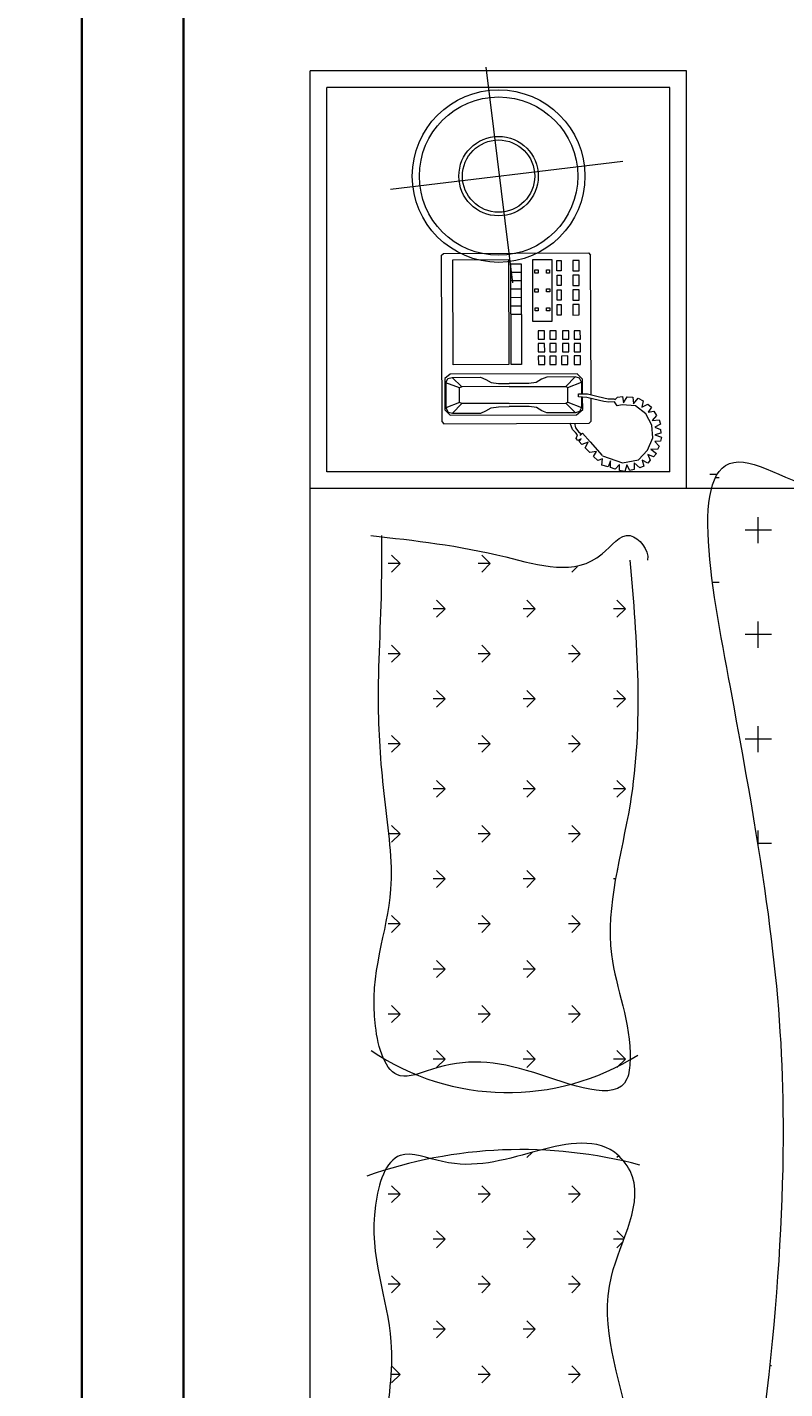
# Model space of a CAD drawing. Units: inches. Extents: x 3731 to 4318, y 1310 to 2388.
# Tile 36 of 57: x 3833 to 3870, y 2243 to 2310. Entities that reach past the tile are written whole.
import ezdxf

# ---------------------------------------------------------------- set-up
doc = ezdxf.new("R2010")
doc.units = ezdxf.units.IN
for name, color, linetype, lineweight in [('A-ANNO-DIMS', 2, 'Continuous', 18), ('A-FURN', 8, 'Continuous', 13), ('A-WALL', 7, 'Continuous', 35)]:
    doc.layers.add(name, color=color, linetype=linetype, lineweight=lineweight)
doc.styles.get("Standard").update_dxf_attribs({"font": 'arial.ttf'})
doc.dimstyles.get("Standard").update_dxf_attribs({"dimtxt": 0.18, "dimasz": 0.18, "dimexe": 0.18, "dimexo": 0.0625, "dimgap": 0.09, "dimtad": 0, "dimtih": 1, "dimtoh": 1, "dimdec": 4, "dimzin": 0, "dimdsep": 46, "dimtxsty": 'Standard', "dimcen": 0.09, "dimadec": 0, "dimazin": 0, "dimtfac": 1, "dimtdec": 4, "dimtofl": 0, "dimtmove": 0, "dimatfit": 3, "dimfxl": 1, "dimtolj": 1, "dimtzin": 0, "dimarcsym": 0})

# ---------------------------------------------------------------- blocks, each defined once
blk = doc.blocks.new('A$C200C7901')
for p, q in [((0.5, 2.3334), (2, 2.3334)), ((2, 2.3334), (2.5, 2.3334)), ((2, 1.6055), (2, 2.3334)), ((2.5, 1.8834), (2.5, 2.3334)), ((0.9943, 2.1721), (0.9842, 2.1822)), ((0.9943, 2.1721), (0.9842, 2.1822)), ((1.3176, 2.1721), (1.3075, 2.1822)), ((1.3176, 2.1721), (1.3075, 2.1822)), ((0.9943, 2.0643), (0.9842, 2.0744)), ((0.9943, 2.0643), (0.9842, 2.0744)), ((1.206, 2.0681), (1.1997, 2.0744)), ((1.206, 2.0681), (1.1997, 2.0744)), ((1.2019, 1.9645), (1.1997, 1.9666)), ((1.2019, 1.9645), (1.1997, 1.9666)), ((2, 1.8834), (2.5, 1.8834)), ((2.0129, 1.8445), (2.0129, 1.849)), ((2.0129, 1.8445), (2.0129, 1.849)), ((2.0171, 1.8467), (2.0171, 1.8556)), ((2.0171, 1.8467), (2.0171, 1.8556))]:
    blk.add_line(p, q)
at = {"linetype": 'ByBlock'}
for p, q in [((2.02, 2.3134), (2.48, 2.3134)), ((2.02, 1.9034), (2.02, 2.3134)), ((2.48, 1.9034), (2.48, 2.3134)), ((0.9404, 2.2259), (0.9303, 2.236)), ((0.9404, 2.2259), (0.9303, 2.236)), ((0.9404, 2.2259), (0.9404, 2.2369)), ((0.9404, 2.2259), (0.9404, 2.2369)), ((0.9404, 2.2259), (0.9505, 2.236)), ((0.9404, 2.2259), (0.9505, 2.236)), ((1.0482, 2.2259), (1.0381, 2.236)), ((1.0482, 2.2259), (1.0381, 2.236)), ((1.0482, 2.2259), (1.0482, 2.2402)), ((1.0482, 2.2259), (1.0482, 2.2402)), ((1.0482, 2.2259), (1.0583, 2.236)), ((1.0482, 2.2259), (1.0583, 2.236)), ((1.1559, 2.2259), (1.1458, 2.236)), ((1.1559, 2.2259), (1.1458, 2.236)), ((1.1559, 2.2259), (1.1559, 2.2402)), ((1.1559, 2.2259), (1.1559, 2.2402)), ((1.1559, 2.2259), (1.166, 2.236)), ((1.1559, 2.2259), (1.166, 2.236)), ((1.3714, 2.2259), (1.3613, 2.236)), ((1.3714, 2.2259), (1.3613, 2.236)), ((1.3714, 2.2259), (1.3714, 2.2402)), ((1.3714, 2.2259), (1.3714, 2.2402)), ((1.3714, 2.2259), (1.3815, 2.236)), ((1.3714, 2.2259), (1.3815, 2.236)), ((1.4792, 2.2259), (1.4691, 2.236)), ((1.4792, 2.2259), (1.4691, 2.236)), ((1.4792, 2.2259), (1.4792, 2.2402)), ((1.4792, 2.2259), (1.4792, 2.2402)), ((1.4792, 2.2259), (1.4893, 2.236)), ((1.4792, 2.2259), (1.4893, 2.236)), ((1.587, 2.2259), (1.5769, 2.236)), ((1.587, 2.2259), (1.5769, 2.236)), ((1.587, 2.2259), (1.587, 2.2393)), ((1.587, 2.2259), (1.587, 2.2393)), ((1.587, 2.2259), (1.5971, 2.236)), ((1.587, 2.2259), (1.5971, 2.236)), ((1.6947, 2.2259), (1.6846, 2.236)), ((1.6947, 2.2259), (1.6846, 2.236)), ((1.6947, 2.2259), (1.6947, 2.2402)), ((1.6947, 2.2259), (1.6947, 2.2402)), ((1.6947, 2.2259), (1.7048, 2.236)), ((1.6947, 2.2259), (1.7048, 2.236)), ((1.8025, 2.2259), (1.7924, 2.236)), ((1.8025, 2.2259), (1.7924, 2.236)), ((1.8025, 2.2259), (1.8025, 2.2402)), ((1.8025, 2.2259), (1.8025, 2.2402)), ((1.8025, 2.2259), (1.8126, 2.236)), ((1.8025, 2.2259), (1.8126, 2.236)), ((1.9103, 2.2259), (1.9002, 2.236)), ((1.9103, 2.2259), (1.9002, 2.236)), ((1.9103, 2.2259), (1.9103, 2.2402)), ((1.9103, 2.2259), (1.9103, 2.2402)), ((1.9103, 2.2259), (1.9204, 2.236)), ((1.9103, 2.2259), (1.9204, 2.236)), ((2.3581, 2.2373), (2.3919, 1.9595)), ((0.9943, 2.172), (0.9943, 2.1863)), ((0.9943, 2.172), (0.9943, 2.1863)), ((1.102, 2.172), (1.102, 2.1863)), ((1.102, 2.172), (1.102, 2.1863)), ((1.3176, 2.172), (1.3176, 2.1863)), ((1.3176, 2.172), (1.3176, 2.1863)), ((1.4253, 2.172), (1.4253, 2.1863)), ((1.4253, 2.172), (1.4253, 2.1863)), ((1.5331, 2.172), (1.5331, 2.1863)), ((1.5331, 2.172), (1.5331, 2.1863)), ((1.6408, 2.172), (1.6408, 2.1863)), ((1.6408, 2.172), (1.6408, 2.1863)), ((1.7486, 2.172), (1.7486, 2.1863)), ((1.7486, 2.172), (1.7486, 2.1863)), ((1.8564, 2.172), (1.8564, 2.1863)), ((1.8564, 2.172), (1.8564, 2.1863)), ((0.9943, 2.1721), (1.0044, 2.1822)), ((0.9943, 2.1721), (1.0044, 2.1822)), ((1.102, 2.1721), (1.0919, 2.1822)), ((1.102, 2.1721), (1.0919, 2.1822)), ((1.102, 2.1721), (1.1121, 2.1822)), ((1.102, 2.1721), (1.1121, 2.1822)), ((1.3176, 2.1721), (1.3277, 2.1822)), ((1.3176, 2.1721), (1.3277, 2.1822)), ((1.4253, 2.1721), (1.4152, 2.1822)), ((1.4253, 2.1721), (1.4152, 2.1822)), ((1.4253, 2.1721), (1.4354, 2.1822)), ((1.4253, 2.1721), (1.4354, 2.1822)), ((1.5331, 2.1721), (1.523, 2.1822)), ((1.5331, 2.1721), (1.523, 2.1822)), ((1.5331, 2.1721), (1.5432, 2.1822)), ((1.5331, 2.1721), (1.5432, 2.1822)), ((1.6409, 2.1721), (1.6308, 2.1822)), ((1.6409, 2.1721), (1.6308, 2.1822)), ((1.6409, 2.1721), (1.651, 2.1822)), ((1.6409, 2.1721), (1.651, 2.1822)), ((1.7486, 2.1721), (1.7385, 2.1822)), ((1.7486, 2.1721), (1.7385, 2.1822)), ((1.7486, 2.1721), (1.7587, 2.1822)), ((1.7486, 2.1721), (1.7587, 2.1822)), ((1.8564, 2.1721), (1.8463, 2.1822)), ((1.8564, 2.1721), (1.8463, 2.1822)), ((1.8564, 2.1721), (1.8665, 2.1822)), ((1.8564, 2.1721), (1.8665, 2.1822)), ((2.0802, 2.176), (2.0777, 2.1734)), ((2.0777, 2.1734), (2.0783, 1.9999)), ((2.2789, 2.1766), (2.0802, 2.176)), ((2.0941, 2.1722), (2.0878, 2.1659)), ((2.0915, 2.1685), (2.0903, 2.1634)), ((2.0966, 2.171), (2.0915, 2.1685)), ((2.1318, 2.1724), (2.0941, 2.1722)), ((2.1267, 2.1711), (2.0966, 2.171)), ((2.1029, 2.1547), (2.0966, 2.171)), ((2.1205, 2.1547), (2.1267, 2.1711)), ((2.1267, 2.1711), (2.1318, 2.1686)), ((2.1368, 2.1661), (2.1318, 2.1724)), ((2.1318, 2.1686), (2.1331, 2.1636)), ((2.2789, 2.1766), (2.2814, 2.1741)), ((2.2814, 2.1741), (2.282, 2.0006)), ((2.0878, 2.1659), (2.0883, 2.015)), ((2.0903, 2.1634), (2.1017, 2.1521)), ((2.0903, 2.1634), (2.0904, 2.1295)), ((2.1017, 2.1521), (2.1029, 2.1547)), ((2.1019, 2.0956), (2.1017, 2.1521)), ((2.1029, 2.1547), (2.1205, 2.1547)), ((2.1218, 2.1522), (2.1205, 2.1547)), ((2.1331, 2.1636), (2.1218, 2.1522)), ((2.122, 2.0956), (2.1218, 2.1522)), ((2.1331, 2.1636), (2.1332, 2.1296)), ((2.1373, 2.014), (2.1368, 2.1661)), ((2.1481, 2.1624), (2.2739, 2.1628)), ((2.1484, 2.0957), (2.1481, 2.1624)), ((2.2739, 2.1628), (2.2741, 2.0961)), ((0.9404, 2.1182), (0.9303, 2.1283)), ((0.9404, 2.1182), (0.9303, 2.1283)), ((0.9404, 2.1182), (0.9404, 2.1325)), ((0.9404, 2.1182), (0.9404, 2.1325)), ((0.9404, 2.1182), (0.9505, 2.1283)), ((0.9404, 2.1182), (0.9505, 2.1283)), ((1.0482, 2.1182), (1.0381, 2.1283)), ((1.0482, 2.1182), (1.0381, 2.1283)), ((1.0482, 2.1182), (1.0482, 2.1325)), ((1.0482, 2.1182), (1.0482, 2.1325)), ((1.0482, 2.1182), (1.0583, 2.1283)), ((1.0482, 2.1182), (1.0583, 2.1283)), ((1.1559, 2.1182), (1.1458, 2.1283)), ((1.1559, 2.1182), (1.1458, 2.1283)), ((1.1559, 2.1182), (1.1559, 2.1325)), ((1.1559, 2.1182), (1.1559, 2.1325)), ((1.1559, 2.1182), (1.166, 2.1283)), ((1.1559, 2.1182), (1.166, 2.1283)), ((1.3714, 2.1182), (1.3613, 2.1283)), ((1.3714, 2.1182), (1.3613, 2.1283)), ((1.3714, 2.1182), (1.3714, 2.1325)), ((1.3714, 2.1182), (1.3714, 2.1325)), ((1.3714, 2.1182), (1.3815, 2.1283)), ((1.3714, 2.1182), (1.3815, 2.1283)), ((1.4792, 2.1182), (1.4691, 2.1283)), ((1.4792, 2.1182), (1.4691, 2.1283)), ((1.4792, 2.1182), (1.4792, 2.1325)), ((1.4792, 2.1182), (1.4792, 2.1325)), ((1.4792, 2.1182), (1.4893, 2.1283)), ((1.4792, 2.1182), (1.4893, 2.1283)), ((1.587, 2.1182), (1.5769, 2.1283)), ((1.587, 2.1182), (1.5769, 2.1283)), ((1.587, 2.1182), (1.587, 2.1325)), ((1.587, 2.1182), (1.587, 2.1325)), ((1.587, 2.1182), (1.5971, 2.1283)), ((1.587, 2.1182), (1.5971, 2.1283)), ((1.6947, 2.1182), (1.6846, 2.1283)), ((1.6947, 2.1182), (1.6846, 2.1283)), ((1.6947, 2.1182), (1.6947, 2.1325)), ((1.6947, 2.1182), (1.6947, 2.1325)), ((1.6947, 2.1182), (1.7048, 2.1283)), ((1.6947, 2.1182), (1.7048, 2.1283)), ((1.8025, 2.1182), (1.7924, 2.1283)), ((1.8025, 2.1182), (1.7924, 2.1283)), ((1.8025, 2.1182), (1.8025, 2.1325)), ((1.8025, 2.1182), (1.8025, 2.1325)), ((1.8025, 2.1182), (1.8126, 2.1283)), ((1.8025, 2.1182), (1.8126, 2.1283)), ((1.9103, 2.1182), (1.9002, 2.1283)), ((1.9103, 2.1182), (1.9002, 2.1283)), ((1.9103, 2.1182), (1.9103, 2.1325)), ((1.9103, 2.1182), (1.9103, 2.1325)), ((1.9103, 2.1182), (1.9204, 2.1283)), ((1.9103, 2.1182), (1.9204, 2.1283)), ((2.0904, 2.1295), (2.093, 2.1232)), ((2.093, 2.1232), (2.0968, 2.1169)), ((2.1307, 2.1233), (2.1269, 2.117)), ((2.1332, 2.1296), (2.1307, 2.1233)), ((2.2464, 2.0911), (2.5044, 2.1228)), ((2.0968, 2.1169), (2.098, 2.1081)), ((2.098, 2.1081), (2.0981, 2.0956)), ((2.1269, 2.117), (2.1257, 2.1082)), ((2.1257, 2.1082), (2.1257, 2.0956)), ((2.0982, 2.0717), (2.0981, 2.0956)), ((2.1019, 2.0956), (2.1021, 2.0277)), ((2.122, 2.0956), (2.1222, 2.0277)), ((2.1258, 2.0718), (2.1257, 2.0956)), ((2.2741, 2.0961), (2.1484, 2.0957)), ((2.1484, 2.0932), (2.2691, 2.0936)), ((2.1484, 2.0806), (2.1484, 2.0932)), ((2.2087, 2.0934), (2.2088, 2.0808)), ((2.2188, 2.0934), (2.2188, 2.0809)), ((2.2288, 2.0935), (2.2289, 2.0809)), ((2.2389, 2.0935), (2.239, 2.0809)), ((2.249, 2.0935), (2.249, 2.081)), ((2.259, 2.0936), (2.2591, 2.081)), ((2.2691, 2.0936), (2.2691, 2.081)), ((0.9943, 2.0643), (0.9943, 2.0786)), ((0.9943, 2.0643), (0.9943, 2.0786)), ((0.9943, 2.0643), (1.0044, 2.0744)), ((0.9943, 2.0643), (1.0044, 2.0744)), ((1.102, 2.0643), (1.0919, 2.0744)), ((1.102, 2.0643), (1.0919, 2.0744)), ((1.102, 2.0643), (1.102, 2.0786)), ((1.102, 2.0643), (1.102, 2.0786)), ((1.102, 2.0643), (1.1121, 2.0744)), ((1.102, 2.0643), (1.1121, 2.0744)), ((1.3176, 2.0643), (1.3075, 2.0744)), ((1.3176, 2.0643), (1.3075, 2.0744)), ((1.3176, 2.0643), (1.3176, 2.0786)), ((1.3176, 2.0643), (1.3176, 2.0786)), ((1.3176, 2.0643), (1.3277, 2.0744)), ((1.3176, 2.0643), (1.3277, 2.0744)), ((1.4253, 2.0643), (1.4152, 2.0744)), ((1.4253, 2.0643), (1.4152, 2.0744)), ((1.4253, 2.0643), (1.4253, 2.0786)), ((1.4253, 2.0643), (1.4253, 2.0786)), ((1.4253, 2.0643), (1.4354, 2.0744)), ((1.4253, 2.0643), (1.4354, 2.0744)), ((1.5331, 2.0643), (1.523, 2.0744)), ((1.5331, 2.0643), (1.523, 2.0744)), ((1.5331, 2.0643), (1.5331, 2.0786)), ((1.5331, 2.0643), (1.5331, 2.0786)), ((1.5331, 2.0643), (1.5432, 2.0744)), ((1.5331, 2.0643), (1.5432, 2.0744)), ((1.6409, 2.0643), (1.6308, 2.0744)), ((1.6409, 2.0643), (1.6308, 2.0744)), ((1.6408, 2.0643), (1.6408, 2.0786)), ((1.6408, 2.0643), (1.6408, 2.0786)), ((1.6409, 2.0643), (1.651, 2.0744)), ((1.6409, 2.0643), (1.651, 2.0744)), ((1.7486, 2.0643), (1.7385, 2.0744)), ((1.7486, 2.0643), (1.7385, 2.0744)), ((1.7486, 2.0643), (1.7486, 2.0786)), ((1.7486, 2.0643), (1.7486, 2.0786)), ((1.7486, 2.0643), (1.7587, 2.0744)), ((1.7486, 2.0643), (1.7587, 2.0744)), ((1.8564, 2.0643), (1.8463, 2.0744)), ((1.8564, 2.0643), (1.8463, 2.0744)), ((1.8564, 2.0643), (1.8564, 2.0786)), ((1.8564, 2.0643), (1.8564, 2.0786)), ((1.8564, 2.0643), (1.8665, 2.0744)), ((1.8564, 2.0643), (1.8665, 2.0744)), ((2.0969, 2.0629), (2.0982, 2.0717)), ((2.1271, 2.063), (2.1258, 2.0718)), ((2.2691, 2.081), (2.1484, 2.0806)), ((2.0907, 2.0503), (2.0932, 2.0566)), ((2.0932, 2.0566), (2.0969, 2.0629)), ((2.1309, 2.0567), (2.1271, 2.063)), ((2.1334, 2.0504), (2.1309, 2.0567)), ((2.1586, 2.0606), (2.1485, 2.0605)), ((2.1485, 2.0605), (2.1485, 2.053)), ((2.1485, 2.053), (2.1586, 2.053)), ((2.1586, 2.053), (2.1586, 2.0606)), ((2.1636, 2.0606), (2.1636, 2.053)), ((2.1736, 2.0606), (2.1636, 2.0606)), ((2.1636, 2.053), (2.1737, 2.0531)), ((2.1737, 2.0531), (2.1736, 2.0606)), ((2.1887, 2.0607), (2.1787, 2.0606)), ((2.1787, 2.0606), (2.1787, 2.0531)), ((2.1787, 2.0531), (2.1888, 2.0531)), ((2.1888, 2.0531), (2.1887, 2.0607)), ((2.2, 2.067), (2.2742, 2.0672)), ((2.2001, 2.0443), (2.2, 2.067)), ((2.2126, 2.0645), (2.2164, 2.0645)), ((2.2126, 2.0607), (2.2126, 2.0645)), ((2.2164, 2.0607), (2.2126, 2.0607)), ((2.2164, 2.0645), (2.2164, 2.0607)), ((2.2352, 2.0646), (2.239, 2.0646)), ((2.2352, 2.0608), (2.2352, 2.0646)), ((2.239, 2.0608), (2.2352, 2.0608)), ((2.239, 2.0646), (2.239, 2.0608)), ((2.2579, 2.0609), (2.2579, 2.0647)), ((2.2579, 2.0647), (2.2616, 2.0647)), ((2.2616, 2.0609), (2.2579, 2.0609)), ((2.2616, 2.0647), (2.2616, 2.0609)), ((2.2742, 2.0672), (2.2743, 2.0446)), ((2.0908, 2.0163), (2.0907, 2.0503)), ((2.1336, 2.0165), (2.1334, 2.0504)), ((2.1485, 2.0467), (2.1486, 2.0391)), ((2.1586, 2.0467), (2.1485, 2.0467)), ((2.1486, 2.0391), (2.1586, 2.0392)), ((2.1586, 2.0392), (2.1586, 2.0467)), ((2.1737, 2.0468), (2.1636, 2.0467)), ((2.1636, 2.0467), (2.1637, 2.0392)), ((2.1637, 2.0392), (2.1737, 2.0392)), ((2.1737, 2.0392), (2.1737, 2.0468)), ((2.1787, 2.0468), (2.1787, 2.0392)), ((2.1888, 2.0468), (2.1787, 2.0468)), ((2.1787, 2.0392), (2.1888, 2.0393)), ((2.1888, 2.0393), (2.1888, 2.0468)), ((2.2743, 2.0446), (2.2001, 2.0443)), ((2.2077, 2.0331), (2.2077, 2.0381)), ((2.2077, 2.0381), (2.2202, 2.0381)), ((2.2126, 2.0507), (2.2164, 2.0507)), ((2.2127, 2.0469), (2.2126, 2.0507)), ((2.2164, 2.0469), (2.2127, 2.0469)), ((2.2164, 2.0507), (2.2164, 2.0469)), ((2.2202, 2.0381), (2.2203, 2.0331)), ((2.2253, 2.0381), (2.2378, 2.0382)), ((2.2253, 2.0331), (2.2253, 2.0381)), ((2.2353, 2.0508), (2.2391, 2.0508)), ((2.2353, 2.047), (2.2353, 2.0508)), ((2.2391, 2.047), (2.2353, 2.047)), ((2.2378, 2.0382), (2.2379, 2.0332)), ((2.2391, 2.0508), (2.2391, 2.047)), ((2.2429, 2.0332), (2.2429, 2.0382)), ((2.2429, 2.0382), (2.2554, 2.0382)), ((2.2554, 2.0382), (2.2555, 2.0332)), ((2.2579, 2.0508), (2.2617, 2.0508)), ((2.2579, 2.0471), (2.2579, 2.0508)), ((2.2617, 2.0471), (2.2579, 2.0471)), ((2.2605, 2.0332), (2.2605, 2.0383)), ((2.2605, 2.0383), (2.273, 2.0383)), ((2.2617, 2.0508), (2.2617, 2.0471)), ((2.273, 2.0383), (2.2731, 2.0333)), ((0.9404, 2.0104), (0.9303, 2.0205)), ((0.9404, 2.0104), (0.9303, 2.0205)), ((0.9404, 2.0104), (0.9404, 2.0247)), ((0.9404, 2.0104), (0.9404, 2.0247)), ((0.9404, 2.0104), (0.9505, 2.0205)), ((0.9404, 2.0104), (0.9505, 2.0205)), ((1.0482, 2.0104), (1.0381, 2.0205)), ((1.0482, 2.0104), (1.0381, 2.0205)), ((1.0482, 2.0104), (1.0482, 2.0247)), ((1.0482, 2.0104), (1.0482, 2.0247)), ((1.0482, 2.0104), (1.0583, 2.0205)), ((1.0482, 2.0104), (1.0583, 2.0205)), ((1.1559, 2.0104), (1.1458, 2.0205)), ((1.1559, 2.0104), (1.1458, 2.0205)), ((1.1559, 2.0104), (1.1559, 2.0247)), ((1.1559, 2.0104), (1.1559, 2.0247)), ((1.1559, 2.0104), (1.166, 2.0205)), ((1.1559, 2.0104), (1.166, 2.0205)), ((1.3714, 2.0104), (1.3613, 2.0205)), ((1.3714, 2.0104), (1.3613, 2.0205)), ((1.3714, 2.0104), (1.3714, 2.0247)), ((1.3714, 2.0104), (1.3714, 2.0247)), ((1.3714, 2.0104), (1.3815, 2.0205)), ((1.3714, 2.0104), (1.3815, 2.0205)), ((1.4792, 2.0104), (1.4691, 2.0205)), ((1.4792, 2.0104), (1.4691, 2.0205)), ((1.4792, 2.0104), (1.4792, 2.0247)), ((1.4792, 2.0104), (1.4792, 2.0247)), ((1.4792, 2.0104), (1.4893, 2.0205)), ((1.4792, 2.0104), (1.4893, 2.0205)), ((1.587, 2.0104), (1.5769, 2.0205)), ((1.587, 2.0104), (1.5769, 2.0205)), ((1.587, 2.0104), (1.587, 2.0247)), ((1.587, 2.0104), (1.587, 2.0247)), ((1.587, 2.0104), (1.5971, 2.0205)), ((1.587, 2.0104), (1.5971, 2.0205)), ((1.6947, 2.0104), (1.6846, 2.0205)), ((1.6947, 2.0104), (1.6846, 2.0205)), ((1.6947, 2.0104), (1.6947, 2.0247)), ((1.6947, 2.0104), (1.6947, 2.0247)), ((1.6947, 2.0104), (1.7048, 2.0205)), ((1.6947, 2.0104), (1.7048, 2.0205)), ((1.8025, 2.0104), (1.7924, 2.0205)), ((1.8025, 2.0104), (1.7924, 2.0205)), ((1.8025, 2.0104), (1.8025, 2.0247)), ((1.8025, 2.0104), (1.8025, 2.0247)), ((1.8025, 2.0104), (1.8126, 2.0205)), ((1.8025, 2.0104), (1.8126, 2.0205)), ((1.9068, 2.0139), (1.9002, 2.0205)), ((1.9068, 2.0139), (1.9002, 2.0205)), ((2.0707, 2.0197), (2.0782, 2.0226)), ((2.0908, 2.0163), (2.1021, 2.0277)), ((2.1034, 2.0252), (2.0971, 2.0088)), ((2.1021, 2.0277), (2.1034, 2.0252)), ((2.1034, 2.0252), (2.121, 2.0252)), ((2.1222, 2.0277), (2.121, 2.0252)), ((2.121, 2.0252), (2.1273, 2.0089)), ((2.1336, 2.0165), (2.1222, 2.0277)), ((2.1586, 2.0329), (2.1486, 2.0329)), ((2.1486, 2.0329), (2.1486, 2.0253)), ((2.1486, 2.0253), (2.1587, 2.0253)), ((2.1587, 2.0253), (2.1586, 2.0329)), ((2.1637, 2.0317), (2.1637, 2.0241)), ((2.1737, 2.0317), (2.1637, 2.0317)), ((2.1637, 2.0241), (2.1738, 2.0241)), ((2.1738, 2.0241), (2.1737, 2.0317)), ((2.1788, 2.0317), (2.1788, 2.0242)), ((2.1888, 2.0317), (2.1788, 2.0317)), ((2.1788, 2.0242), (2.1889, 2.0242)), ((2.1889, 2.0242), (2.1888, 2.0317)), ((2.2203, 2.0331), (2.2077, 2.0331)), ((2.2379, 2.0332), (2.2253, 2.0331)), ((2.2555, 2.0332), (2.2429, 2.0332)), ((2.2731, 2.0333), (2.2605, 2.0332)), ((2.0431, 1.999), (2.0488, 2.0046)), ((2.0488, 2.0046), (2.0557, 2.0011)), ((2.053, 2.0084), (2.0563, 2.0119)), ((2.0557, 2.0011), (2.053, 2.0084)), ((2.0663, 2.0077), (2.0561, 1.9986)), ((2.0563, 2.0119), (2.0594, 2.0095)), ((2.0576, 2.0133), (2.0598, 2.0155)), ((2.0594, 2.0095), (2.0576, 2.0133)), ((2.0598, 2.0155), (2.0645, 2.0137)), ((2.0663, 2.0102), (2.0636, 2.0104)), ((2.0636, 2.0104), (2.0663, 2.0077)), ((2.0645, 2.0137), (2.0671, 2.0162)), ((2.0676, 2.012), (2.0663, 2.0102)), ((2.0671, 2.0162), (2.0707, 2.0197)), ((2.0727, 2.016), (2.0676, 2.012)), ((2.0782, 2.0175), (2.0727, 2.016)), ((2.0883, 2.015), (2.0946, 2.0075)), ((2.0921, 2.0113), (2.0908, 2.0163)), ((2.0971, 2.0088), (2.0921, 2.0113)), ((2.0946, 2.0075), (2.1093, 2.0076)), ((2.1094, 2.0088), (2.0971, 2.0088)), ((2.109, 2.0025), (2.1097, 2.0126)), ((2.1097, 2.0126), (2.1135, 2.0126)), ((2.1135, 2.0126), (2.1133, 2.0018)), ((2.1273, 2.0089), (2.1134, 2.0088)), ((2.1134, 2.0076), (2.1311, 2.0077)), ((2.1273, 2.0089), (2.1323, 2.0114)), ((2.1311, 2.0077), (2.1373, 2.014)), ((2.1323, 2.0114), (2.1336, 2.0165)), ((2.1587, 2.0178), (2.1486, 2.0178)), ((2.1486, 2.0178), (2.1487, 2.0102)), ((2.1487, 2.0102), (2.1587, 2.0103)), ((2.1587, 2.0103), (2.1587, 2.0178)), ((2.1738, 2.0179), (2.1637, 2.0178)), ((2.1637, 2.0178), (2.1638, 2.0103)), ((2.1638, 2.0103), (2.1738, 2.0103)), ((2.1738, 2.0103), (2.1738, 2.0179)), ((2.1788, 2.0179), (2.1788, 2.0103)), ((2.1889, 2.0179), (2.1788, 2.0179)), ((2.1788, 2.0103), (2.1889, 2.0104)), ((2.1889, 2.0104), (2.1889, 2.0179)), ((2.2203, 2.0193), (2.2077, 2.0192)), ((2.2077, 2.0192), (2.2078, 2.0117)), ((2.2078, 2.0117), (2.2203, 2.0117)), ((2.2203, 2.0117), (2.2203, 2.0193)), ((2.2379, 2.0193), (2.2253, 2.0193)), ((2.2253, 2.0193), (2.2254, 2.0117)), ((2.2254, 2.0117), (2.2379, 2.0118)), ((2.2379, 2.0118), (2.2379, 2.0193)), ((2.2555, 2.0194), (2.2429, 2.0193)), ((2.2429, 2.0193), (2.243, 2.0118)), ((2.243, 2.0118), (2.2555, 2.0118)), ((2.2555, 2.0118), (2.2555, 2.0194)), ((2.2605, 2.0194), (2.2606, 2.0119)), ((2.2731, 2.0194), (2.2605, 2.0194)), ((2.2606, 2.0119), (2.2731, 2.0119)), ((2.2731, 2.0119), (2.2731, 2.0194)), ((2.0338, 1.9895), (2.0386, 1.9946)), ((2.0358, 1.9839), (2.0338, 1.9895)), ((2.0386, 1.9946), (2.0444, 1.9911)), ((2.0561, 1.9986), (2.0396, 1.9844)), ((2.0444, 1.9911), (2.0431, 1.999)), ((2.0783, 1.9999), (2.0808, 1.9974)), ((2.0808, 1.9974), (2.1079, 1.9975)), ((2.1042, 1.9824), (2.1072, 1.9944)), ((2.1072, 1.9944), (2.109, 2.0025)), ((2.1103, 1.989), (2.1073, 1.9771)), ((2.1133, 2.0018), (2.1103, 1.989)), ((2.1123, 1.9975), (2.2795, 1.9981)), ((2.282, 2.0006), (2.2795, 1.9981)), ((2.0234, 1.9686), (2.0251, 1.9745)), ((2.0251, 1.9745), (2.0333, 1.9743)), ((2.0259, 1.977), (2.0281, 1.9847)), ((2.0333, 1.9743), (2.0259, 1.977)), ((2.0281, 1.9847), (2.0358, 1.9839)), ((2.0393, 1.984), (2.031, 1.96)), ((2.1035, 1.9763), (2.1042, 1.9824)), ((2.1038, 1.9697), (2.1035, 1.9763)), ((2.1073, 1.9771), (2.1076, 1.9704)), ((1.0993, 1.9593), (1.0919, 1.9666)), ((1.0993, 1.9593), (1.0919, 1.9666)), ((1.102, 1.9583), (1.102, 1.9708)), ((1.102, 1.9583), (1.102, 1.9708)), ((1.1033, 1.9578), (1.1121, 1.9666)), ((1.1033, 1.9578), (1.1121, 1.9666)), ((1.3176, 1.9565), (1.3075, 1.9666)), ((1.3176, 1.9565), (1.3075, 1.9666)), ((1.3176, 1.9565), (1.3176, 1.9708)), ((1.3176, 1.9565), (1.3176, 1.9708)), ((1.3176, 1.9565), (1.3277, 1.9666)), ((1.3176, 1.9565), (1.3277, 1.9666)), ((1.4253, 1.9703), (1.4253, 1.9708)), ((1.4253, 1.9703), (1.4253, 1.9708)), ((1.5331, 1.9683), (1.5331, 1.9708)), ((1.5331, 1.9683), (1.5331, 1.9708)), ((1.543, 1.9665), (1.5432, 1.9666)), ((1.543, 1.9665), (1.5432, 1.9666)), ((1.6409, 1.9565), (1.6308, 1.9666)), ((1.6409, 1.9565), (1.6308, 1.9666)), ((1.6408, 1.9565), (1.6408, 1.9708)), ((1.6408, 1.9565), (1.6408, 1.9708)), ((1.6409, 1.9565), (1.651, 1.9666)), ((1.6409, 1.9565), (1.651, 1.9666)), ((1.7486, 1.9565), (1.7385, 1.9666)), ((1.7486, 1.9565), (1.7385, 1.9666)), ((1.7486, 1.9565), (1.7486, 1.9708)), ((1.7486, 1.9565), (1.7486, 1.9708)), ((1.7486, 1.9565), (1.7587, 1.9666)), ((1.7486, 1.9565), (1.7587, 1.9666)), ((1.8564, 1.9565), (1.8463, 1.9666)), ((1.8564, 1.9565), (1.8463, 1.9666)), ((1.8564, 1.9565), (1.8564, 1.9708)), ((1.8564, 1.9565), (1.8564, 1.9708)), ((1.8564, 1.9565), (1.8665, 1.9666)), ((1.8564, 1.9565), (1.8665, 1.9666)), ((2.0206, 1.9572), (2.0218, 1.9635)), ((2.0285, 1.9549), (2.0206, 1.9572)), ((2.0218, 1.9635), (2.0287, 1.9636)), ((2.0219, 1.9511), (2.0285, 1.9549)), ((2.0287, 1.9636), (2.0234, 1.9686)), ((2.031, 1.96), (2.0346, 1.9409)), ((2.099, 1.9444), (2.1002, 1.9605)), ((2.0992, 1.9663), (2.1038, 1.9697)), ((2.1002, 1.9605), (2.0992, 1.9663)), ((2.1101, 1.96), (2.1028, 1.9587)), ((2.1028, 1.9587), (2.1099, 1.9544)), ((2.1076, 1.9704), (2.1068, 1.9689)), ((2.1068, 1.9689), (2.1096, 1.9661)), ((2.1096, 1.9661), (2.1101, 1.96)), ((2.0229, 1.946), (2.0219, 1.9511)), ((2.0308, 1.9462), (2.0229, 1.946)), ((2.0247, 1.9394), (2.0308, 1.9462)), ((2.0268, 1.9343), (2.0247, 1.9394)), ((2.0346, 1.9409), (2.0459, 1.93)), ((2.0894, 1.9322), (2.099, 1.9444)), ((2.1094, 1.9475), (2.1013, 1.9467)), ((2.1013, 1.9467), (2.1084, 1.9412)), ((2.1084, 1.9412), (2.1051, 1.9353)), ((2.1099, 1.9544), (2.1094, 1.9475)), ((2.0341, 1.9366), (2.0268, 1.9343)), ((2.0306, 1.9297), (2.0341, 1.9366)), ((2.0339, 1.9267), (2.0306, 1.9297)), ((2.041, 1.9297), (2.0339, 1.9267)), ((2.038, 1.9228), (2.041, 1.9297)), ((2.0421, 1.9193), (2.038, 1.9228)), ((2.0474, 1.9259), (2.0421, 1.9193)), ((2.0459, 1.93), (2.0607, 1.9237)), ((2.0467, 1.9183), (2.0474, 1.9259)), ((2.0607, 1.9237), (2.0759, 1.925)), ((2.0759, 1.925), (2.0894, 1.9322)), ((2.0876, 1.9195), (2.0815, 1.9245)), ((2.0815, 1.9245), (2.0823, 1.9161)), ((2.0925, 1.9225), (2.0876, 1.9195)), ((2.0973, 1.9251), (2.0914, 1.9294)), ((2.0914, 1.9294), (2.0925, 1.9225)), ((2.1011, 1.9297), (2.0973, 1.9251)), ((2.1051, 1.9353), (2.0975, 1.9368)), ((2.0975, 1.9368), (2.1011, 1.9297)), ((2.0508, 1.9163), (2.0467, 1.9183)), ((2.0566, 1.9214), (2.0508, 1.9163)), ((2.0569, 1.9145), (2.0566, 1.9214)), ((2.0617, 1.9133), (2.0569, 1.9145)), ((2.0645, 1.9214), (2.0617, 1.9133)), ((2.0663, 1.914), (2.0645, 1.9214)), ((2.0706, 1.9146), (2.0663, 1.914)), ((2.0736, 1.9214), (2.0706, 1.9146)), ((2.077, 1.9146), (2.0736, 1.9214)), ((2.0823, 1.9161), (2.077, 1.9146)), ((2.02, 1.9034), (2.48, 1.9034)), ((1.8879, 1.8445), (1.8879, 1.8523)), ((1.8879, 1.8445), (1.8879, 1.8523)), ((1.7004, 1.782), (1.7004, 1.8133)), ((1.7004, 1.782), (1.7004, 1.8133)), ((1.8254, 1.782), (1.8254, 1.8133)), ((1.8254, 1.782), (1.8254, 1.8133)), ((1.9504, 1.782), (1.9504, 1.8133)), ((1.9504, 1.782), (1.9504, 1.8133)), ((1.573, 1.7977), (1.591, 1.7977)), ((1.573, 1.7977), (1.591, 1.7977)), ((1.5754, 1.782), (1.5754, 1.7981)), ((1.5754, 1.782), (1.5754, 1.7981)), ((1.6847, 1.7977), (1.716, 1.7977)), ((1.6847, 1.7977), (1.716, 1.7977)), ((1.8097, 1.7977), (1.841, 1.7977)), ((1.8097, 1.7977), (1.841, 1.7977)), ((1.9347, 1.7977), (1.966, 1.7977)), ((1.9347, 1.7977), (1.966, 1.7977)), ((0.9504, 1.782), (0.9504, 1.7836)), ((0.9504, 1.782), (0.9504, 1.7836))]:
    blk.add_line(p, q, dxfattribs=at)
for radius in [0.1032, 0.0947, 0.0475, 0.0432]:
    blk.add_circle((2.3739, 2.1081), radius, dxfattribs=at)
for centre, radius, start, end in [((0.658, 2.0811), 0.5513, 345.0722, 19.5492), ((1.5685, 2.097), 0.291, 145.8603, 212.2445)]:
    blk.add_arc(centre, radius, start, end)
for points, knots in [([(0.5854, 1.951), (0.6835, 1.9407), (0.8425, 1.9242), (1.0374, 2.0054), (1.1564, 1.9255), (1.2274, 1.9841), (1.2052, 2.0751), (1.1815, 2.152), (1.2176, 2.2368), (1.0992, 2.2731), (1.0008, 2.2255), (0.8698, 2.246), (0.7481, 2.2548), (0.6426, 2.2473), (0.5746, 2.2478), (0.5562, 2.2479)], [0, 0, 0, 0, 292.165466, 473.33038, 601.631673, 630.723769, 727.138505, 836.819956, 887.958136, 954.42438, 1118.989809, 1227.016542, 1338.750986, 1487.447361, 1542.751028, 1542.751028, 1542.751028, 1542.751028]), ([(1.9146, 1.951), (1.8174, 1.9428), (1.6601, 1.9297), (1.4574, 1.9942), (1.3549, 1.9462), (1.2593, 1.9563), (1.314, 2.0834), (1.3193, 2.1569), (1.2853, 2.2393), (1.4031, 2.2724), (1.4987, 2.2256), (1.6304, 2.2459), (1.7519, 2.2548), (1.8574, 2.2473), (1.9254, 2.2478), (1.9438, 2.2479)], [0, 0, 0, 0, 292.165466, 473.33038, 601.631673, 624.236147, 735.870502, 858.452188, 896.317728, 962.783971, 1127.3494, 1235.376134, 1347.110578, 1495.806953, 1551.11062, 1551.11062, 1551.11062, 1551.11062]), ([(1.9438, 2.2608), (1.9381, 2.2086), (1.9282, 2.1195), (1.8897, 2.0022), (1.9591, 1.9538), (1.9264, 1.9278), (1.9146, 1.93)], [0, 0, 0, 0, 163.411291, 278.570782, 318.445997, 354.484131, 354.484131, 354.484131, 354.484131]), ([(0.4485, 1.7835), (0.4321, 1.7496), (0.4062, 1.6964), (0.49, 1.6713), (0.4719, 1.5969), (0.4123, 1.592), (0.4233, 1.5337), (0.4954, 1.5086), (0.4012, 1.4738), (0.3253, 1.4306), (0.4113, 1.3764), (0.3688, 1.3065), (0.5579, 1.2663), (0.741, 1.4533), (1.1127, 1.1109), (1.4811, 1.2478), (1.7885, 1.3492), (2.0357, 1.1637), (2.0748, 1.2974), (2.0876, 1.349), (2.0192, 1.3805), (2.0564, 1.4298), (2.0588, 1.4846), (1.9759, 1.5349), (2.1004, 1.5845), (2.0397, 1.6519), (1.971, 1.7053), (2.1104, 1.8981), (1.5946, 1.7967), (1.2448, 1.7472), (0.8129, 1.7935), (0.4953, 1.8548), (0.4582, 1.7983), (0.4485, 1.7835)], [0, 0, 0, 0, 88.420092, 139.08588, 204.302936, 239.695496, 287.801042, 327.365471, 412.960499, 463.626286, 552.059846, 584.668336, 662.614915, 940.993281, 1309.926334, 1844.022653, 1996.276242, 2316.43048, 2341.441004, 2404.707416, 2449.463774, 2514.680778, 2538.40571, 2613.031547, 2697.13096, 2760.903931, 2822.692699, 2945.47, 3215.060018, 3725.584917, 4361.974444, 4504.671998, 4555.32777, 4555.32777, 4555.32777, 4555.32777])]:
    blk.add_open_spline(points, degree=3, knots=knots)
blk = doc.blocks.new('*D33')
at = {"layer": 'A-ANNO-DIMS', "color": 0, "lineweight": -2, "transparency": 16777216}
for p, q in [((3835.146, 2338.382), (3731.412, 2338.382)), ((3731.592, 2338.202), (3731.592, 1849.063)), ((3731.592, 1359.562), (3731.592, 1848.7)), ((3835.146, 1359.382), (3731.412, 1359.382))]:
    blk.add_line(p, q, dxfattribs=at)
at = {"layer": 'A-ANNO-DIMS', "color": 0, "transparency": 16777216}
for points in [[(3731.562, 2338.202), (3731.622, 2338.202), (3731.592, 2338.382)], [(3731.562, 1359.562), (3731.622, 1359.562), (3731.592, 1359.382)]]:
    blk.add_solid(points, dxfattribs=at)
at = {"layer": 'Defpoints', "color": 0, "transparency": 16777216}
for p in [(3731.592, 2338.382), (3835.209, 2338.382), (3835.209, 1359.382)]:
    blk.add_point(p, dxfattribs=at)
at = {"layer": 'A-ANNO-DIMS', "color": 0, "transparency": 16777216, "insert": (3731.592, 1848.882), "char_height": 0.18, "attachment_point": 5}
blk.add_mtext('\\A1;979', dxfattribs=at)

msp = doc.modelspace()

# ---------------------------------------------------------------- linework, layer by layer
at = {"layer": 'A-WALL'}
for p, q in [((3835.209, 2338.382), (3835.209, 1359.382)), ((3840.209, 2333.382), (3840.209, 2156.382))]:
    msp.add_line(p, q, dxfattribs=at)

# ---------------------------------------------------------------- block references
at = {"layer": 'A-FURN', "xscale": 41.1071563136412, "yscale": 41.1071563136412, "zscale": 41.1071563136412, "rotation": 90}
msp.add_blockref('A$C200C7901', (3942.346, 2204.601), dxfattribs=at)

# ---------------------------------------------------------------- dimensions: what is measured, and where the dimension line sits
at = {"layer": 'A-ANNO-DIMS'}
dim = msp.add_linear_dim(base=(3731.592, 2338.382), p1=(3835.209, 1359.382), p2=(3835.209, 2338.382), angle=90, dimstyle='Standard', override={"dimdec": 0, "dimlfac": 1, "dimrnd": 0, "dimzin": 0, "dimdsep": 46, "dimlunit": 2}, dxfattribs=at)
dim.commit()
dim.dimension.update_dxf_attribs({"geometry": '*D33', "text_midpoint": (3731.592, 1848.882)})

doc.saveas('drawing.dxf')
